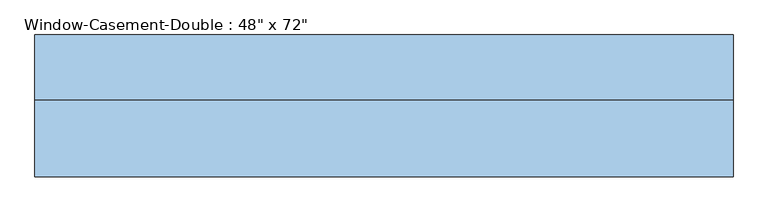
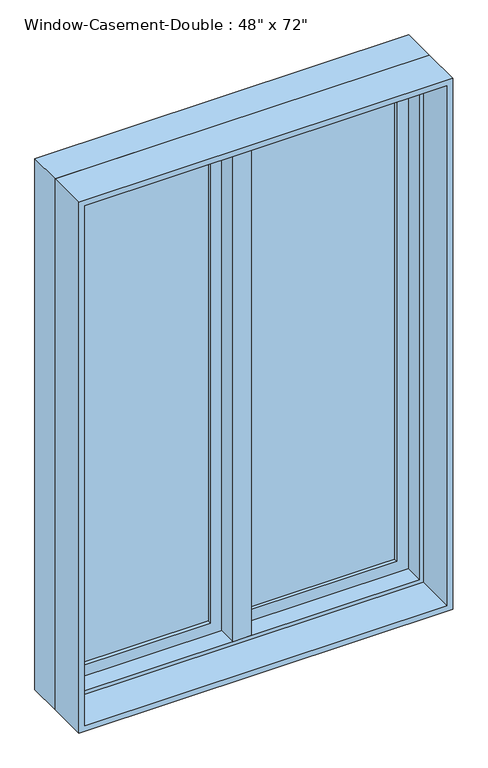
"""IFC4 building model written with IfcOpenShell, lengths in millimetres: window geometry."""

from ifc_helpers import new_model, si_unit, frame, origin, place, context, project, spatial, polyline, outline, extrude, faceted_brep, source, transform, mapped, element, save


def window_6ca1769e(model_context):
    return source(origin(), model_context, "Body", "SolidModel", [
        faceted_brep([(9.525, 133.35, 2730.5), (-9.525, 133.35, 2730.5), (-9.525, 82.55, 2730.5), (9.525, 82.55, 2730.5), (9.525, 133.35, 927.1), (9.525, 82.55, 927.1), (-9.525, 82.55, 927.1), (-9.525, 133.35, 927.1), (-9.525, 82.55, 946.15), (-9.525, 82.55, 2711.45), (-30.1625, 82.55, 946.15), (-30.1625, 82.55, 2711.45), (-30.1625, 19.05, 946.15), (-30.1625, 19.05, 2711.45), (30.1625, 19.05, 946.15), (30.1625, 19.05, 2711.45), (30.1625, 82.55, 946.15), (30.1625, 82.55, 2711.45), (9.525, 82.55, 946.15), (9.525, 82.55, 2711.45)], [[[0, 1, 2, 3]], [[4, 5, 6, 7]], [[1, 0, 4, 7]], [[2, 1, 7, 6, 8, 9]], [[9, 8, 10, 11]], [[11, 10, 12, 13]], [[13, 12, 14, 15]], [[15, 14, 16, 17]], [[17, 16, 18, 19]], [[0, 3, 19, 18, 5, 4]], [[18, 8, 6, 5]], [[9, 19, 3, 2]], [[8, 18, 16, 14, 12, 10]], [[19, 9, 11, 13, 15, 17]]]),
        extrude(outline(polyline([(-66.675, 114.3), (-66.675, 107.95), (-539.75, 107.95), (-539.75, 114.3), (-66.675, 114.3)])), frame((0.0, 0.0, 984.25), z_axis=(0.0, 0.0, 1.0), x_axis=(1.0, 0.0, 0.0)), (0.0, 0.0, 1.0), 1689.1),
        extrude(outline(polyline([(-539.75, 95.25), (-539.75, 101.6), (-66.675, 101.6), (-66.675, 95.25), (-539.75, 95.25)])), frame((0.0, 0.0, 984.25), z_axis=(0.0, 0.0, 1.0), x_axis=(1.0, 0.0, 0.0)), (0.0, 0.0, 1.0), 1689.1),
        extrude(outline(polyline([(539.75, 114.3), (539.75, 107.95), (66.675, 107.95), (66.675, 114.3), (539.75, 114.3)])), frame((0.0, 0.0, 984.25), z_axis=(0.0, 0.0, 1.0), x_axis=(1.0, 0.0, 0.0)), (0.0, 0.0, 1.0), 1689.1),
        extrude(outline(polyline([(66.675, 95.25), (66.675, 101.6), (539.75, 101.6), (539.75, 95.25), (66.675, 95.25)])), frame((0.0, 0.0, 984.25), z_axis=(0.0, 0.0, 1.0), x_axis=(1.0, 0.0, 0.0)), (0.0, 0.0, 1.0), 1689.1),
        extrude(outline(polyline([(2730.5, -596.9), (927.1, -596.9), (927.1, -9.525), (2730.5, -9.525), (2730.5, -596.9)]), holes=[polyline([(2673.35, -66.675), (984.25, -66.675), (984.25, -539.75), (2673.35, -539.75), (2673.35, -66.675)])]), frame((0.0, 82.55, 0.0), z_axis=(0.0, 1.0, 0.0), x_axis=(0.0, 0.0, 1.0)), (0.0, 0.0, 1.0), 44.45),
        extrude(outline(polyline([(927.1, 596.9), (2730.5, 596.9), (2730.5, 9.525), (927.1, 9.525), (927.1, 596.9)]), holes=[polyline([(984.25, 66.675), (2673.35, 66.675), (2673.35, 539.75), (984.25, 539.75), (984.25, 66.675)])]), frame((0.0, 82.55, 0.0), z_axis=(0.0, 1.0, 0.0), x_axis=(0.0, 0.0, 1.0)), (0.0, 0.0, 1.0), 44.45),
        extrude(outline(polyline([(2743.2, -609.6), (914.4, -609.6), (914.4, 609.6), (2743.2, 609.6), (2743.2, -609.6)]), holes=[polyline([(2724.15, 590.55), (933.45, 590.55), (933.45, -590.55), (2724.15, -590.55), (2724.15, 590.55)])]), frame((0.0, -114.3, 0.0), z_axis=(0.0, 1.0, 0.0), x_axis=(0.0, 0.0, 1.0)), (0.0, 0.0, 1.0), 133.35),
        faceted_brep([(577.85, 82.55, 2711.45), (577.85, 19.05, 2711.45), (-577.85, 19.05, 2711.45), (-577.85, 82.55, 2711.45), (596.9, 133.35, 2730.5), (596.9, 82.55, 2730.5), (-596.9, 82.55, 2730.5), (-596.9, 133.35, 2730.5), (609.6, 19.05, 2743.2), (609.6, 133.35, 2743.2), (-609.6, 133.35, 2743.2), (-609.6, 19.05, 2743.2), (-577.85, 19.05, 946.15), (-577.85, 82.55, 946.15), (-596.9, 82.55, 927.1), (-596.9, 133.35, 927.1), (-609.6, 133.35, 914.4), (-609.6, 19.05, 914.4), (577.85, 19.05, 946.15), (577.85, 82.55, 946.15), (596.9, 82.55, 927.1), (596.9, 133.35, 927.1), (609.6, 133.35, 914.4), (609.6, 19.05, 914.4)], [[[0, 1, 2, 3]], [[4, 5, 6, 7]], [[8, 9, 10, 11]], [[3, 2, 12, 13]], [[7, 6, 14, 15]], [[11, 10, 16, 17]], [[13, 12, 18, 19]], [[15, 14, 20, 21]], [[17, 16, 22, 23]], [[11, 17, 23, 8], [1, 18, 12, 2]], [[19, 18, 1, 0]], [[5, 20, 14, 6], [3, 13, 19, 0]], [[21, 20, 5, 4]], [[23, 22, 9, 8]], [[9, 22, 16, 10], [7, 15, 21, 4]]]),
    ])


if __name__ == "__main__":
    model = new_model("IFC4")
    model_context = context("Model", 3, world=origin())
    ifc_project = project(units=[si_unit("LENGTHUNIT", "METRE", prefix="MILLI")], contexts=[model_context])
    site = spatial("IfcSite", under=ifc_project)
    building = spatial("IfcBuilding", under=site)
    placement = place(None, origin())
    window_shape = window_6ca1769e(model_context)
    element("IfcWindow", 1, ObjectType="Window-Casement-Double : 48\" x 72\"", at=placement, inside=building, context=model_context, shape_type="MappedRepresentation", body=[
        mapped(window_shape, transform((0.0, 0.0, 0.0), x_axis=(1.0, 0.0, 0.0), y_axis=(0.0, 1.0, 0.0), z_axis=(0.0, 0.0, 1.0))),
    ])
    save(model, "model.ifc")

# Revit data of these elements
# Type "Window-Casement-Double : 48\" x 72\""
#   Type Mark = "17"
#   Fire Rating = "0.5h"
#   Assembly Code = "B2020100"
#   Analytic Construction = "Double glazing - domestic"
#   Frame Extension [instance default] = 0' - 0 1/4"
#   Window Inset [instance default] = 0' - 0"
#   Wall Thickness [instance default] = 0' - 6"
#   Interior Wall Closure [instance default] = 0' - 2 1/4"
#   Half Width = 2' - 0"
#   Visual Light Transmittance = 0.81
#   Thermal Resistance (R) = 1.8146 (h·ft²·°F)/BTU
#   Solar Heat Gain Coefficient = 0.76
#   Rough Width = 4' - 0 1/2"
#   Rough Height = 6' - 0 1/2"
#   Height = 6' - 0"
#   Heat Transfer Coefficient (U) = 0.5511 BTU/(h·ft²·°F)
#   Exterior Wall Closure [instance default] = 0' - 1 1/4"
#   Extension Jamb [instance default] = 0' - 2 1/4"
#   Default Sill Height = 3' - 0"
#   Width = 4' - 0"
#   Define Thermal Properties by = 0
#   Muntin Visibility = yes
#   Interior Trim Visibility [instance default] = yes
#   Exterior Trim Visibility [instance default] = yes
#   Extension Jamb Visibility [instance default] = yes
#   Interior Trim Material = Wood - Stained
#   Muntin Pattern = Muntin Pattern_2x2 : Muntin Pattern_2x2
#   Interior Trim = Trim-Window-Interior-Flat : Picture Frame
#   Interior Frame Material = Wood - Stained
#   Glass Panel Material = Glass
#   Exterior Trim Material = Clad - White
#   Exterior Trim = Trim-Window-Exterior-Flat : with Sill
#   Exterior Frame Material = Clad - White
#   Wall Closure = (empty or 0)
# Element 1 (IfcWindow, "Window-Casement-Double : 48\" x 72\"")
#   Wall Thickness = 0' - 9"
#   Extension Jamb = 0' - 5 1/4"
#   Materials on its faces: "Wood - Stained", "Glass", "Clad - White"
# Materials
#   "Wood - Stained": class "Wood", colour RGB 224 178 126, transparency 0, Cost = 0
#   "Glass": class "Glass", colour RGB 0 128 192, transparency 0.75, Description = "Soda Lime Glass", Cost = 0
#   "Clad - White": class "Wood", colour RGB 242 242 238, transparency 0, Cost = 0
